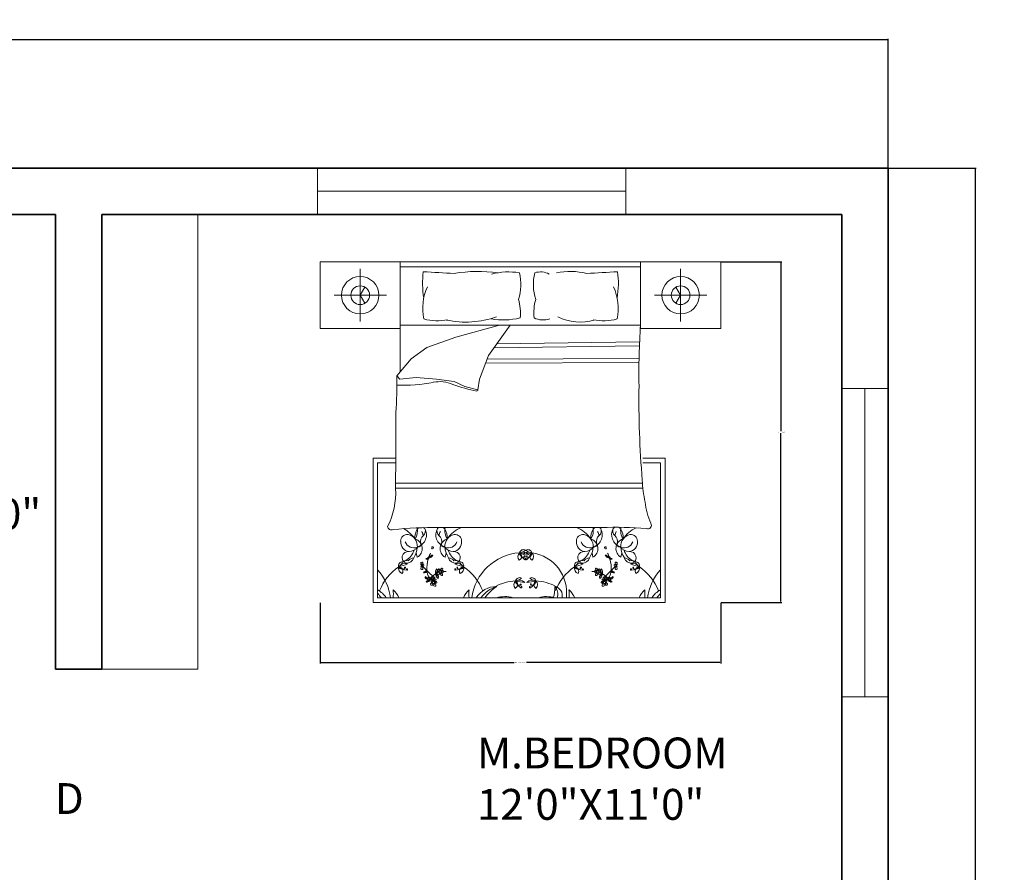
# Model space of a CAD drawing. Units: inches. Extents: x -43 to 1296, y -568 to 542.
# Tile 4 of 14: x 220 to 411, y -130 to 36. Entities that reach past the tile are written whole.
import ezdxf

# ---------------------------------------------------------------- set-up
doc = ezdxf.new("R2010")
doc.units = ezdxf.units.IN
doc.header["$MEASUREMENT"] = 0
for name, color, linetype, lineweight in [('A-ANNO-DIMS', 2, 'Continuous', 18), ('A-ANNO-TEXT', 7, 'Continuous', 18), ('A-AREA-IDEN', 7, 'Continuous', 18), ('A-FLOR-CASE', 9, 'Continuous', 18), ('A-FURN', 8, 'Continuous', 13), ('A-GLAZ', 6, 'Continuous', 18), ('A-WALL', 7, 'Continuous', 35)]:
    doc.layers.add(name, color=color, linetype=linetype, lineweight=lineweight)
doc.styles.get("Standard").update_dxf_attribs({"font": 'arial.ttf'})
doc.dimstyles.get("Standard").update_dxf_attribs({"dimtxt": 0.18, "dimasz": 0.18, "dimexe": 0.18, "dimexo": 0.0625, "dimgap": 0.09, "dimtad": 0, "dimtih": 1, "dimtoh": 1, "dimdec": 0, "dimzin": 0, "dimdsep": 46, "dimlunit": 3, "dimtxsty": 'Standard', "dimcen": 0.09, "dimadec": 0, "dimazin": 0, "dimtfac": 1, "dimtdec": 0, "dimtofl": 0, "dimtmove": 0, "dimatfit": 3, "dimfxl": 1, "dimtolj": 1, "dimtzin": 0, "dimarcsym": 0})

# ---------------------------------------------------------------- blocks, each defined once
blk = doc.blocks.new('*D1')
at = {"layer": 'A-ANNO-DIMS', "color": 0, "lineweight": -2, "transparency": 16777216}
for p, q in [((28.84, 6.72), (28.84, 31.8)), ((29.02, 31.62), (203.66, 31.62)), ((388.66, 31.62), (214.02, 31.62)), ((388.84, 6.72), (388.84, 31.8))]:
    blk.add_line(p, q, dxfattribs=at)
at = {"layer": 'A-ANNO-DIMS', "color": 0, "transparency": 16777216}
for points in [[(29.02, 31.65), (29.02, 31.59), (28.84, 31.62)], [(388.66, 31.65), (388.66, 31.59), (388.84, 31.62)]]:
    blk.add_solid(points, dxfattribs=at)
at = {"layer": 'Defpoints', "color": 0, "transparency": 16777216}
for p in [(388.84, 31.62), (28.84, 6.66), (388.84, 6.66)]:
    blk.add_point(p, dxfattribs=at)
at = {"layer": 'A-ANNO-DIMS', "color": 0, "transparency": 16777216, "insert": (208.84, 31.62), "char_height": 6, "attachment_point": 5}
blk.add_mtext("\\A1;30'", dxfattribs=at)
blk = doc.blocks.new('*D2')
at = {"layer": 'A-ANNO-DIMS', "color": 0, "lineweight": -2, "transparency": 16777216}
for p, q in [((388.91, 6.66), (405.97, 6.66)), ((405.79, 6.48), (405.79, -230.19)), ((405.79, -473.16), (405.79, -236.49)), ((388.91, -473.34), (405.97, -473.34))]:
    blk.add_line(p, q, dxfattribs=at)
at = {"layer": 'A-ANNO-DIMS', "color": 0, "transparency": 16777216}
for points in [[(405.76, 6.48), (405.82, 6.48), (405.79, 6.66)], [(405.76, -473.16), (405.82, -473.16), (405.79, -473.34)]]:
    blk.add_solid(points, dxfattribs=at)
at = {"layer": 'Defpoints', "color": 0, "transparency": 16777216}
for p in [(388.84, 6.66), (388.84, -473.34), (405.79, -473.34)]:
    blk.add_point(p, dxfattribs=at)
at = {"layer": 'A-ANNO-DIMS', "color": 0, "transparency": 16777216, "insert": (405.79, -233.34), "char_height": 6, "attachment_point": 5}
blk.add_mtext("\\A1;40'", dxfattribs=at)
blk = doc.blocks.new('BED-SUITE-78')
for p, q in [((0, 66.29), (77.95, 66.29)), ((15.59, 66.29), (15.59, 44.89)), ((62.36, 65.29), (15.59, 65.29)), ((7.79, 54.7), (7.79, 64.89)), ((70.15, 54.7), (70.15, 64.89)), ((12.89, 59.79), (2.7, 59.79)), ((65.06, 59.79), (75.25, 59.79)), ((15.59, 53.97), (62.36, 53.97)), ((26.42, 51.65), (34.92, 53.97)), ((37, 53.97), (32.73, 48.03)), ((20.73, 49.6), (26.42, 51.65)), ((62.12, 49.93), (33.82, 49.53)), ((62.15, 50.73), (34.4, 50.34)), ((17.73, 47.39), (20.73, 49.6)), ((32.73, 48.03), (31, 43.45)), ((14.89, 44.08), (17.73, 47.39)), ((62.08, 46.68), (32.17, 46.56)), ((62.08, 47.48), (32.48, 47.36)), ((15.52, 43.45), (14.89, 44.08)), ((18.68, 43.77), (15.52, 43.45)), ((22.63, 43.45), (18.68, 43.77)), ((26.1, 42.98), (22.63, 43.45)), ((28.15, 42.03), (26.1, 42.98)), ((31, 43.45), (30.68, 41.4)), ((30.68, 41.4), (28.15, 42.03)), ((10.29, 28.08), (14.7, 28.08)), ((10.29, 0), (10.29, 28.08)), ((14.7, 27.18), (11.19, 27.18)), ((11.19, 27.18), (11.19, 0.9)), ((66.21, 27.18), (62.78, 27.18)), ((62.79, 28.08), (67.12, 28.08)), ((66.21, 0.9), (66.21, 27.18)), ((67.12, 28.08), (67.12, 0)), ((62.71, 23.22), (14.69, 23.22)), ((62.79, 22.25), (14.69, 22.25)), ((54.8, 14.59), (23.15, 14.59)), ((18.87, 8.81), (18.7, 9.69)), ((24.32, 8.81), (24.49, 9.69)), ((53.08, 8.81), (52.91, 9.69)), ((58.53, 8.81), (58.7, 9.69)), ((67.12, 0), (10.29, 0)), ((11.19, 0.9), (66.21, 0.9))]:
    blk.add_line(p, q)
for points in [[(15.59, 53.3), (0, 53.3), (0, 66.29)], [(62.36, 66.29), (62.36, 53.3), (77.95, 53.3), (77.95, 66.29)], [(7.79, 59.79), (8.7, 61.37)], [(70.15, 59.79), (69.24, 61.37)], [(7.79, 59.79), (8.7, 58.22)], [(70.15, 59.79), (69.24, 58.22)]]:
    blk.add_lwpolyline(points)
for points in [[(20.07, 64.35, 0.074897), (20.16, 59.26, -0.472817)], [(38.61, 58.97, 0.14099), (38.76, 64.16, 0.235245)], [(41.94, 58.97, -0.14099), (41.78, 64.16, -0.235245)], [(57.88, 64.35, -0.074897), (57.79, 59.26, 0.472817)], [(14.73, 36.94, 0.001242), (14.69, 22.15, -0.127202), (13.13, 14.78)], [(62.69, 23.83, 0.056112), (63.26, 19.54, 0.095341), (64.35, 15.41)]]:
    blk.add_lwpolyline(points, format="xyb")
for centre, radius in [((7.79, 59.79), 3.64), ((70.15, 59.79), 3.64), ((7.79, 59.79), 1.82), ((70.15, 59.79), 1.82), ((23.38, 5.98), 0.199), ((54.03, 5.98), 0.199), ((22.08, 3.89), 0.199), ((55.33, 3.89), 0.199)]:
    blk.add_circle(centre, radius)
for centre, radius, start, end in [((63.03, 806.15), 743.04, 266.68521, 267.14978), ((30.75, 36.14), 28.27, 82.2196, 99.497), ((36.72, 50.43), 13.89, 81.5249, 103.96), ((42.85, 60.46), 3.86, 63.3437, 106.1026), ((48.63, 50.71), 13.7, 76.3427, 101.1841), ((14.92, 806.15), 743.04, 272.85022, 273.31479), ((30, 57.21), 10.05, 155.1316, 191.7583), ((47.95, 57.21), 10.05, 348.2417, 24.8684), ((29.42, 56.37), 9.55, 354.0129, 15.8293), ((51.13, 56.37), 9.55, 164.1707, 185.9871), ((28.35, 72.68), 18.12, 258.0397, 289.2615), ((50.59, 64.49), 9.92, 243.8761, 286.1746), ((22.85, 65.26), 10.45, 255.1039, 281.0369), ((35.68, 68.73), 13.75, 259.8617, 283.6238), ((43.37, 59.11), 4.13, 245.0183, 288.5407), ((55.1, 65.26), 10.45, 258.9631, 284.8961), ((202.09, 44.45), 140.06, 176.1, 180.9282), ((-56.58, 42.14), 71.5, 355.8294, 1.553), ((16.23, 71.68), 29.42, 267.4519, 281.3392), ((23.26, 36.62), 6.35, 66.2616, 101.3392), ((36.09, 70.85), 30.23, 250.1194, 259.3383), ((244.73, 39.35), 182.7, 179.1145, 184.8735), ((30.5, 41.34), 0.188, 268.8623, 19.7536), ((63.76, 15.02), 0.71, 246.5219, 33.8264), ((13.85, 14.83), 0.719, 183.98, 297.3412), ((22.22, -66.55), 81.14, 89.3433, 95.6887), ((13.54, 9.1), 5.9, 33.6671, 63.2997), ((21.45, 12.61), 3.01, 145.785, 184.7304), ((15.71, 14.01), 3.23, 328.8218, 9.1554), ((19.71, 13.73), 0.939, 120.0293, 142.325), ((18.21, 13.17), 2.48, 289.2822, 29.1751), ((17.83, 12.72), 2.24, 7.436, 29.9149), ((19.31, 13.91), 1.17, 311.5653, 23.8354), ((19.71, 13.73), 0.939, 44.4517, 63.558), ((24.99, 13.17), 2.48, 150.8249, 250.7178), ((23.88, 13.91), 1.17, 156.1646, 228.4347), ((23.49, 13.73), 0.939, 113.229, 135.5483), ((25.36, 12.72), 2.24, 150.0851, 172.564), ((23.49, 13.73), 0.939, 37.675, 66.7144), ((21.74, 12.61), 3.01, 355.2696, 34.215), ((27.49, 14.01), 3.23, 169.7133, 211.1782), ((29.65, 9.1), 5.9, 111.4941, 146.3329), ((47.75, 9.1), 5.9, 33.6671, 68.5059), ((55.66, 12.61), 3.01, 145.785, 184.7304), ((49.92, 14.01), 3.23, 328.8218, 10.2867), ((53.92, 13.73), 0.939, 113.2856, 142.325), ((52.42, 13.17), 2.48, 289.2822, 29.1751), ((52.04, 12.72), 2.24, 7.436, 29.9149), ((53.92, 13.73), 0.939, 44.4517, 66.7144), ((53.52, 13.91), 1.17, 311.5653, 23.8354), ((57.18, -61.22), 75.85, 85.2402, 91.8035), ((59.2, 13.17), 2.48, 150.8249, 250.7178), ((58.09, 13.91), 1.17, 156.1646, 228.4347), ((57.7, 13.73), 0.939, 106.6343, 135.5483), ((59.57, 12.72), 2.24, 150.0851, 172.564), ((57.7, 13.73), 0.939, 37.675, 72.5814), ((55.96, 12.61), 3.01, 355.2696, 34.215), ((61.7, 14.01), 3.23, 169.249, 211.1782), ((63.86, 9.1), 5.9, 113.6453, 146.3329), ((16.98, 11.93), 1.32, 84.4856, 181.0538), ((17.52, 11.74), 1.86, 174.9449, 262.8857), ((18.25, 12.45), 1.81, 201.5819, 291.4221), ((16.58, 10.96), 2.34, 355.2933, 76.921), ((17.91, 10.49), 1.94, 299.9085, 73.1337), ((21.14, 11.84), 1.6, 131.5653, 195.1471), ((22.05, 11.84), 1.6, 344.8529, 48.4347), ((25.29, 10.49), 1.94, 106.8663, 240.0915), ((26.62, 10.96), 2.34, 103.079, 184.7067), ((24.94, 12.45), 1.81, 248.5779, 338.4181), ((25.68, 11.74), 1.86, 277.1143, 5.0551), ((26.21, 11.93), 1.32, 358.9462, 95.5144), ((51.19, 11.93), 1.32, 84.4856, 181.0538), ((51.73, 11.74), 1.86, 174.9449, 262.8857), ((52.46, 12.45), 1.81, 201.5819, 291.4221), ((50.79, 10.96), 2.34, 355.2933, 76.921), ((52.12, 10.49), 1.94, 299.9085, 73.1337), ((55.35, 11.84), 1.6, 131.5653, 195.1471), ((56.26, 11.84), 1.6, 344.8529, 48.4347), ((59.5, 10.49), 1.94, 106.8663, 240.0915), ((60.83, 10.96), 2.34, 103.079, 184.7067), ((59.15, 12.45), 1.81, 248.5779, 338.4181), ((59.89, 11.74), 1.86, 277.1143, 5.0551), ((60.42, 11.93), 1.32, 358.9462, 95.5144), ((17.09, 8.74), 1.17, 80.264, 250.8688), ((14.77, 11.32), 3.68, 301.2614, 341.7045), ((17.19, 12.16), 2.26, 272.3591, 324.0401), ((14.74, 11.02), 4.18, 326.2883, 356.5076), ((21.45, 12.61), 3.01, 212.7011, 216.3445), ((19.13, 11.3), 0.484, 257.3041, 15.1471), ((21.82, 10.57), 0.15, 102.7051, 280.4384), ((21.8, 10.66), 0.244, 280.4384, 100.4136), ((24.06, 11.3), 0.484, 164.8529, 282.6959), ((21.74, 12.61), 3.01, 323.6555, 327.2989), ((26, 12.16), 2.26, 215.9599, 267.6409), ((28.46, 11.02), 4.18, 183.4924, 213.7117), ((28.42, 11.32), 3.68, 198.2955, 238.7386), ((26.1, 8.74), 1.17, 289.1312, 99.736), ((39.58, -0.47), 10.18, 94.4623, 172.255), ((39.62, 8.92), 1.13, 137.7873, 219.1145), ((38.34, 8.96), 0.85, 298.5391, 58.3627), ((39.6, 9.44), 0.844, 63.0274, 163.8037), ((38.74, 11.42), 1.74, 271.4585, 315.3727), ((39.45, 8.21), 1.61, 45.5411, 114.3101), ((40.92, 16.47), 7.12, 252.593, 267.2582), ((39.62, 9.65), 0.833, 177.7585, 283.852), ((41.22, 10.51), 2.57, 198.9159, 238.011), ((40.55, 8.21), 1.61, 65.6899, 134.4589), ((39.08, 16.47), 7.12, 272.7418, 287.407), ((40.4, 9.44), 0.844, 16.1963, 116.9726), ((41.26, 11.42), 1.74, 224.6273, 268.5415), ((38.78, 10.51), 2.57, 301.989, 341.0841), ((40.38, 9.65), 0.833, 256.148, 2.2415), ((41.66, 8.96), 0.85, 121.6373, 241.4609), ((40.38, 8.92), 1.13, 320.8855, 42.2127), ((40.09, 1.88), 7.88, 352.8636, 81.8197), ((51.3, 8.74), 1.17, 80.264, 250.8688), ((48.98, 11.32), 3.68, 301.2614, 341.7045), ((51.4, 12.16), 2.26, 272.3591, 324.0401), ((48.95, 11.02), 4.18, 326.2883, 356.5076), ((55.66, 12.61), 3.01, 212.7011, 216.3445), ((53.34, 11.3), 0.484, 257.3041, 15.1471), ((55.6, 10.66), 0.244, 79.5864, 259.5616), ((55.58, 10.57), 0.15, 259.5616, 77.2949), ((58.27, 11.3), 0.484, 164.8529, 282.6959), ((55.96, 12.61), 3.01, 323.6555, 327.2989), ((60.21, 12.16), 2.26, 215.9599, 267.6409), ((62.67, 11.02), 4.18, 183.4924, 213.7117), ((62.63, 11.32), 3.68, 198.2955, 238.7386), ((60.31, 8.74), 1.17, 289.1312, 99.736), ((16.1, 7.13), 0.844, 92.9516, 193.728), ((14.37, 8.41), 1.74, 301.3827, 345.2969), ((16.85, 7.48), 0.717, 63.9755, 143.2681), ((16.81, 9.09), 1.46, 265.969, 344.3045), ((18.38, 7.15), 1.56, 96.1662, 141.5825), ((19.8, 7.47), 0.331, 101.5637, 142.6358), ((19.54, 7.73), 0.477, 288.7263, 352.5032), ((19.86, 7.7), 0.153, 345.2356, 144.9248), ((20.96, 8.24), 0.409, 101.3256, 154.4621), ((20.37, 9.63), 1.23, 280.2588, 300.656), ((20.65, 10.62), 2.2, 268.3264, 277.1302), ((27.22, 6.64), 6.46, 163.5842, 183.8277), ((20.1, 9.63), 1.25, 308.2101, 316.3071), ((20.87, 8.81), 0.374, 278.3432, 4.2869), ((20.67, 9.14), 0.653, 300.656, 332.6341), ((21.16, 8.7), 0.159, 55.7657, 157.4417), ((27.22, 6.64), 6.46, 153.0032, 159.8941), ((21.4, 8.85), 0.159, 84.3784, 186.0543), ((21.26, 9.49), 0.653, 269.1859, 301.164), ((21.45, 9.15), 0.374, 237.5332, 323.4768), ((21.08, 10.22), 1.25, 285.5129, 293.6099), ((20.96, 9.98), 1.23, 301.164, 321.5612), ((21.9, 8.81), 0.409, 87.3579, 140.4944), ((19.95, 10.2), 2.2, 324.6898, 333.4936), ((24.81, 7.15), 1.56, 38.4175, 83.8338), ((26.38, 9.09), 1.46, 195.6955, 274.031), ((26.34, 7.48), 0.717, 36.7319, 116.0245), ((27.09, 7.13), 0.844, 346.272, 87.0484), ((28.82, 8.41), 1.74, 194.7031, 238.6173), ((39.79, 8.95), 0.11, 283.852, 219.9245), ((39.93, 8.44), 0.126, 238.011, 71.5592), ((39.95, 8.5), 0.0614, 71.5592, 188.0167), ((40.08, 8.44), 0.126, 108.4408, 301.989), ((40.06, 8.5), 0.0614, 351.9833, 108.4408), ((40.2, 8.99), 0.0664, 320.1909, 256.0209), ((50.31, 7.13), 0.844, 92.9516, 193.728), ((48.58, 8.41), 1.74, 301.3827, 345.2969), ((51.06, 7.48), 0.717, 63.9755, 143.2681), ((51.02, 9.09), 1.46, 265.969, 344.3045), ((52.59, 7.15), 1.56, 96.1662, 141.5825), ((56.45, 9.98), 1.23, 218.4388, 238.836), ((55.5, 8.81), 0.409, 39.5056, 92.6421), ((57.45, 10.2), 2.2, 206.5064, 215.3102), ((55.96, 9.15), 0.374, 216.5232, 302.4668), ((56.15, 9.49), 0.653, 238.836, 270.8141), ((56.32, 10.22), 1.25, 246.3901, 254.4871), ((50.18, 6.64), 6.46, 20.1059, 26.9968), ((56, 8.85), 0.159, 353.9457, 95.6216), ((56.25, 8.7), 0.159, 22.5583, 124.2343), ((56.53, 8.81), 0.374, 175.7131, 261.6568), ((56.74, 9.14), 0.653, 207.3659, 239.344), ((50.18, 6.64), 6.46, 356.1723, 16.4158), ((57.3, 9.63), 1.25, 223.6929, 231.7899), ((57.03, 9.63), 1.23, 239.344, 259.7412), ((56.75, 10.62), 2.2, 262.8698, 271.6736), ((56.44, 8.24), 0.409, 25.5379, 78.6744), ((57.54, 7.7), 0.153, 35.0752, 194.7644), ((57.87, 7.73), 0.477, 187.4968, 251.2737), ((57.6, 7.47), 0.331, 37.3642, 78.4363), ((60.59, 9.09), 1.46, 195.6955, 274.031), ((59.02, 7.15), 1.56, 38.4175, 83.8338), ((60.55, 7.48), 0.717, 36.7319, 116.0245), ((63.03, 8.41), 1.74, 194.7031, 238.6173), ((61.3, 7.13), 0.844, 346.272, 87.0484), ((3.61, -0.47), 10.18, 7.745, 41.8856), ((21.03, -1.47), 10.18, 124.3865, 158.5908), ((16.38, 6.69), 1.13, 167.7115, 249.0387), ((16.59, 5.98), 1.61, 75.4653, 144.2343), ((13.74, 13.88), 7.12, 282.5173, 297.1824), ((15.25, 6.08), 0.85, 328.4633, 88.2869), ((16.97, 8.86), 2.57, 228.8402, 267.9352), ((16.02, 7.31), 0.833, 207.6827, 313.7762), ((16.52, 6.79), 0.11, 313.7762, 249.7183), ((16.87, 6.48), 0.0614, 101.4834, 217.9409), ((16.89, 6.42), 0.126, 267.9352, 101.4834), ((19.53, 7.16), 0.199, 273.2768, 86.7232), ((19.8, 6.79), 0.328, 217.7621, 259.0403), ((19.76, 7.35), 0.19, 91.1081, 181.8675), ((20.15, 7.23), 0.603, 203.4276, 227.6104), ((19.96, 6.97), 0.41, 80.3487, 133.6538), ((19.89, 7.31), 0.325, 229.7889, 317.6792), ((19.52, 6.62), 0.461, 355.053, 68.3618), ((19.88, 6.54), 0.65, 83.0852, 105.7171), ((19.83, 6.59), 0.152, 232.4737, 355.053), ((15.38, 1.15), 7.4, 43.1541, 52.0459), ((20, 7.2), 0.171, 317.6792, 80.3487), ((20.5, 5.62), 0.409, 101.3256, 154.4621), ((19.91, 7.01), 1.23, 280.2588, 300.656), ((20.19, 8), 2.2, 268.3264, 277.1302), ((19.64, 7.01), 1.25, 308.2101, 316.3071), ((20.41, 6.18), 0.374, 278.3432, 4.2869), ((20.2, 6.51), 0.653, 300.656, 332.6341), ((20.69, 6.08), 0.159, 55.7657, 157.4417), ((24.01, 6.48), 3.24, 184.756, 209.2041), ((28.67, 13.37), 10.65, 222.2412, 232.1744), ((21.86, 6.28), 0.905, 304.5369, 16.3699), ((22.34, 6.07), 0.55, 272.8499, 356.1226), ((21.95, 5.86), 0.533, 321.7607, 7.9252), ((23.11, 6.02), 0.64, 127.3105, 187.9252), ((22.23, 6.09), 0.657, 355.0106, 41.658), ((24.34, 2.18), 3.88, 113.0501, 113.8477), ((23.32, 5.38), 0.626, 104.7558, 148.0499), ((22.97, 5.83), 0.392, 247.4086, 351.4386), ((23.16, 6.26), 0.271, 126.1046, 271.4281), ((23.13, 6.33), 0.194, 353.7526, 131.7054), ((23.08, 5.81), 0.131, 262.906, 7.132), ((22.94, 6.1), 0.273, 0.0645, 61.1507), ((23.01, 6.33), 0.312, 311.8413, 355.7877), ((23.65, 6.29), 0.331, 101.5637, 176.365), ((23.65, 5.61), 0.328, 151.2196, 259.0403), ((23.61, 6.17), 0.19, 91.1081, 181.8675), ((24, 6.05), 0.603, 203.4276, 227.6104), ((23.81, 5.79), 0.41, 80.3487, 133.6538), ((23.74, 6.13), 0.325, 229.7889, 317.6792), ((23.38, 6.55), 0.477, 288.7263, 352.5032), ((23.37, 5.44), 0.461, 355.053, 68.3618), ((23.73, 5.36), 0.65, 83.0852, 105.7171), ((23.71, 6.53), 0.153, 345.2356, 144.9248), ((23.85, 6.02), 0.171, 317.6792, 80.3487), ((24.34, 2.18), 3.88, 87.1071, 94.7585), ((26.31, 6.42), 0.126, 78.5166, 272.0648), ((26.61, 5.98), 1.61, 35.7657, 104.5347), ((29.46, 13.88), 7.12, 242.8176, 257.4827), ((26.22, 8.86), 2.57, 272.0648, 311.1598), ((26.32, 6.48), 0.0614, 322.0591, 78.5166), ((27.18, 7.31), 0.833, 226.2238, 332.3173), ((26.69, 6.83), 0.0664, 290.2667, 226.2271), ((27.94, 6.08), 0.85, 91.7131, 211.5367), ((26.81, 6.69), 1.13, 290.9613, 12.2885), ((22.17, -1.47), 10.18, 21.4092, 55.6135), ((55.24, -1.47), 10.18, 124.3865, 158.5908), ((50.59, 6.69), 1.13, 167.7115, 249.0387), ((50.8, 5.98), 1.61, 75.4653, 144.2343), ((47.95, 13.88), 7.12, 282.5173, 297.1824), ((50.23, 7.31), 0.833, 207.6827, 313.7762), ((51.18, 8.86), 2.57, 228.8402, 267.9352), ((49.46, 6.08), 0.85, 328.4633, 88.2869), ((50.73, 6.79), 0.11, 313.7762, 249.7183), ((51.08, 6.48), 0.0614, 101.4834, 217.9409), ((51.1, 6.42), 0.126, 267.9352, 101.4834), ((53.06, 2.18), 3.88, 85.2415, 92.8929), ((53.55, 6.02), 0.171, 99.6513, 222.3208), ((53.67, 6.13), 0.325, 222.3208, 310.2111), ((53.59, 5.79), 0.41, 46.3462, 99.6513), ((53.69, 6.53), 0.153, 35.0752, 194.7644), ((54.02, 6.55), 0.477, 187.4968, 251.2737), ((54.03, 5.44), 0.461, 111.6382, 184.947), ((53.67, 5.36), 0.65, 74.2829, 96.9148), ((53.8, 6.17), 0.19, 358.1325, 88.8919), ((53.4, 6.05), 0.603, 312.3896, 336.5724), ((53.75, 6.29), 0.331, 3.635, 78.4363), ((53.76, 5.61), 0.328, 280.9597, 28.7804), ((54.43, 5.83), 0.392, 188.5614, 292.5914), ((54.28, 6.33), 0.194, 48.2946, 186.2474), ((54.39, 6.33), 0.312, 184.2123, 228.1587), ((54.46, 6.1), 0.273, 118.8493, 179.9355), ((54.32, 5.81), 0.131, 172.868, 277.094), ((54.25, 6.26), 0.271, 268.5719, 53.8954), ((54.08, 5.38), 0.626, 31.9501, 75.2442), ((55.17, 6.09), 0.657, 138.342, 184.9894), ((55.06, 6.07), 0.55, 183.8774, 267.1501), ((53.06, 2.18), 3.88, 66.1523, 66.9499), ((55.55, 6.28), 0.905, 163.6301, 235.4631), ((54.29, 6.02), 0.64, 352.0748, 52.6895), ((55.45, 5.86), 0.533, 172.0748, 218.2393), ((48.74, 13.37), 10.65, 307.8256, 317.7588), ((53.4, 6.48), 3.24, 330.7959, 355.244), ((62.02, 1.15), 7.4, 127.9541, 136.8459), ((56.71, 6.08), 0.159, 22.5583, 124.2343), ((57, 6.18), 0.374, 175.7131, 261.6568), ((57.2, 6.51), 0.653, 207.3659, 239.344), ((57.76, 7.01), 1.25, 223.6929, 231.7899), ((57.5, 7.01), 1.23, 239.344, 259.7412), ((57.21, 8), 2.2, 262.8698, 271.6736), ((56.91, 5.62), 0.409, 25.5379, 78.6744), ((57.4, 7.2), 0.171, 99.6513, 222.3208), ((57.52, 7.31), 0.325, 222.3208, 310.2111), ((57.44, 6.97), 0.41, 46.3462, 99.6513), ((57.88, 6.62), 0.461, 111.6382, 184.947), ((57.57, 6.59), 0.152, 184.947, 307.5263), ((57.52, 6.54), 0.65, 74.2829, 96.9148), ((57.64, 7.35), 0.19, 358.1325, 88.8919), ((57.25, 7.23), 0.603, 312.3896, 336.5724), ((57.61, 6.79), 0.328, 280.9597, 322.2379), ((57.88, 7.16), 0.199, 93.2768, 266.7232), ((60.52, 6.42), 0.126, 78.5166, 272.0648), ((60.82, 5.98), 1.61, 35.7657, 104.5347), ((63.67, 13.88), 7.12, 242.8176, 257.4827), ((60.43, 8.86), 2.57, 272.0648, 311.1598), ((60.53, 6.48), 0.0614, 322.0591, 78.5166), ((61.39, 7.31), 0.833, 226.2238, 332.3173), ((60.9, 6.83), 0.0664, 290.2667, 226.2271), ((62.15, 6.08), 0.85, 91.7131, 211.5367), ((61.02, 6.69), 1.13, 290.9613, 12.2885), ((56.38, -1.47), 10.18, 21.4092, 55.6135), ((73.79, -0.47), 10.18, 138.1144, 172.255), ((20.63, 4.9), 0.222, 146.8636, 236.9021), ((23.76, 9.79), 5.8, 235.1882, 238.8844), ((21.01, 5.22), 0.6, 199.4799, 267.6828), ((20.95, 5), 0.517, 212.8155, 277.3992), ((20.65, 4.65), 0.6, 266.9701, 338.2913), ((17.48, 8.93), 5.8, 302.6784, 306.3746), ((20.8, 4.18), 0.222, 214.3538, 304.3923), ((20.88, 5.02), 0.229, 238.8844, 314.2646), ((20.83, 4.5), 0.517, 280.3057, 17.1958), ((20.79, 4.45), 0.229, 306.3746, 21.7548), ((21.16, 4.6), 0.173, 19.3605, 201.7548), ((21.16, 4.73), 0.173, 311.8703, 134.2646), ((24.42, 3.15), 3.46, 153.7819, 158.2913), ((21.66, 5.51), 0.905, 247.2305, 319.0635), ((21.37, 5.21), 0.533, 264.4544, 310.6188), ((24.01, 6.48), 3.24, 214.0033, 222.4917), ((21.76, 5), 0.55, 218.3208, 298.8162), ((24.34, 2.18), 3.88, 120.544, 139.818), ((22.02, 3.29), 0.626, 104.7558, 148.0499), ((21.86, 4.17), 0.271, 126.1046, 271.4281), ((21.83, 4.24), 0.194, 353.7526, 131.7054), ((22.13, 4.32), 0.64, 70.0041, 130.6188), ((21.65, 4.01), 0.273, 0.0645, 61.1507), ((21.71, 4.24), 0.312, 311.8413, 355.7877), ((21.71, 5.1), 0.657, 297.7043, 344.3516), ((22.35, 4.2), 0.331, 101.5637, 176.365), ((22.31, 4.08), 0.19, 91.1081, 181.8675), ((22.51, 3.7), 0.41, 80.3487, 133.6538), ((22.09, 4.46), 0.477, 288.7263, 352.5032), ((22.43, 3.27), 0.65, 83.0852, 105.7171), ((22.41, 4.43), 0.153, 345.2356, 144.9248), ((22.06, 5.1), 0.533, 8.7227, 54.8872), ((22.09, 4.67), 0.905, 0.278, 72.111), ((22.5, 5), 0.55, 20.5253, 88.5375), ((22.55, 3.93), 0.171, 317.6792, 80.3487), ((23.22, 5.27), 0.64, 188.7227, 249.3375), ((22.96, 5.61), 0.197, 148.0499, 225.6268), ((22.4, 4.95), 0.657, 334.9899, 21.6373), ((23.68, 5.41), 0.152, 232.4737, 355.053), ((38.8, -5.92), 10.18, 94.4623, 117.4146), ((38.84, 3.47), 1.13, 137.7873, 219.1145), ((37.56, 3.5), 0.85, 298.5391, 58.3627), ((38.82, 3.99), 0.844, 63.0274, 163.8037), ((37.96, 5.97), 1.74, 271.4585, 315.3727), ((38.67, 2.76), 1.61, 45.5411, 114.3101), ((40.44, 5.06), 2.57, 198.9159, 238.011), ((40.14, 11.02), 7.12, 252.593, 267.2582), ((38.84, 4.2), 0.833, 177.7585, 283.852), ((41.33, 2.76), 1.61, 65.6899, 134.4589), ((39.86, 11.02), 7.12, 272.7418, 287.407), ((41.18, 3.99), 0.844, 16.1963, 116.9726), ((42.04, 5.97), 1.74, 224.6273, 268.5415), ((39.56, 5.06), 2.57, 301.989, 341.0841), ((41.16, 4.2), 0.833, 256.148, 2.2415), ((42.44, 3.5), 0.85, 121.6373, 241.4609), ((41.16, 3.47), 1.13, 320.8855, 42.2127), ((41.2, -5.92), 10.18, 62.5854, 85.5377), ((53.73, 5.41), 0.152, 184.947, 307.5263), ((55, 4.95), 0.657, 158.3627, 205.0101), ((54.91, 5), 0.55, 91.4625, 159.4747), ((55.31, 4.67), 0.905, 107.889, 179.722), ((54.18, 5.27), 0.64, 290.6625, 351.2773), ((54.44, 5.61), 0.197, 314.3732, 31.9501), ((54.85, 3.93), 0.171, 99.6513, 222.3208), ((55.34, 5.1), 0.533, 125.1128, 171.2773), ((54.89, 3.7), 0.41, 46.3462, 99.6513), ((54.99, 4.43), 0.153, 35.0752, 194.7644), ((55.32, 4.46), 0.477, 187.4968, 251.2737), ((54.97, 3.27), 0.65, 74.2829, 96.9148), ((53.06, 2.18), 3.88, 40.182, 59.456), ((55.27, 4.32), 0.64, 49.3812, 109.9959), ((55.74, 5.51), 0.905, 220.9365, 292.7695), ((55.69, 5.1), 0.657, 195.6484, 242.2957), ((55.09, 4.08), 0.19, 358.1325, 88.8919), ((55.05, 4.2), 0.331, 3.635, 78.4363), ((55.65, 5), 0.55, 241.1838, 321.6792), ((55.58, 4.24), 0.194, 48.2946, 186.2474), ((55.69, 4.24), 0.312, 184.2123, 228.1587), ((55.76, 4.01), 0.273, 118.8493, 179.9355), ((55.55, 4.17), 0.271, 268.5719, 53.8954), ((55.38, 3.29), 0.626, 31.9501, 75.2442), ((56.04, 5.21), 0.533, 229.3812, 275.5456), ((53.4, 6.48), 3.24, 317.5083, 325.9967), ((56.57, 4.5), 0.517, 162.8042, 259.6943), ((56.24, 4.73), 0.173, 45.7354, 228.1297), ((56.24, 4.6), 0.173, 338.2452, 160.6395), ((52.99, 3.15), 3.46, 21.7087, 26.2181), ((56.76, 4.65), 0.6, 201.7087, 273.0299), ((56.52, 5.02), 0.229, 225.7354, 301.1156), ((56.46, 5), 0.517, 262.6008, 327.1845), ((56.62, 4.45), 0.229, 158.2452, 233.6254), ((56.39, 5.22), 0.6, 272.3172, 340.5201), ((59.92, 8.93), 5.8, 233.6254, 237.3216), ((56.61, 4.18), 0.222, 235.6077, 325.6462), ((53.65, 9.79), 5.8, 301.1156, 304.8118), ((56.77, 4.9), 0.222, 303.0979, 33.1364), ((8.72, -1.83), 4.96, 33.4617, 60.1116), ((11.5, -0.68), 4.14, 22.5547, 48.9546), ((0.16, 1.54), 14.08, 357.4081, 3.6519), ((21.66, 3.52), 0.197, 148.0499, 225.6268), ((21.67, 3.74), 0.392, 247.4086, 351.4386), ((21.78, 3.72), 0.131, 262.906, 7.132), ((22.35, 3.52), 0.328, 151.2196, 259.0403), ((22.7, 3.96), 0.603, 203.4276, 227.6104), ((22.44, 4.04), 0.325, 229.7889, 317.6792), ((22.07, 3.35), 0.461, 355.053, 68.3618), ((22.38, 3.32), 0.152, 232.4737, 355.053), ((31.7, -0.68), 4.14, 131.0454, 157.4453), ((43.03, 1.54), 14.08, 176.3481, 182.5919), ((34.47, -1.83), 4.96, 91.272, 146.5383), ((36.26, -2.76), 6.18, 107.8504, 143.6964), ((39.51, -4.49), 9.19, 124.0123, 144.053), ((39.01, 3.49), 0.11, 283.852, 219.9245), ((39.15, 2.99), 0.126, 238.011, 71.5592), ((39.17, 3.05), 0.0614, 71.5592, 188.0167), ((40.86, 2.99), 0.126, 108.4408, 301.989), ((40.83, 3.05), 0.0614, 351.9833, 108.4408), ((40.98, 3.54), 0.0664, 320.1909, 256.0209), ((41.11, 2.6), 4.56, 338.117, 6.6195), ((45.29, 1.33), 1.83, 346.3898, 79.0739), ((43.92, 1.58), 2.31, 342.8609, 41.9049), ((34.37, 1.54), 14.08, 357.4081, 3.6519), ((45.71, -0.68), 4.14, 22.5547, 48.9546), ((54.97, 4.04), 0.325, 222.3208, 310.2111), ((55.33, 3.35), 0.461, 111.6382, 184.947), ((55.03, 3.32), 0.152, 184.947, 307.5263), ((54.7, 3.96), 0.603, 312.3896, 336.5724), ((55.06, 3.52), 0.328, 280.9597, 28.7804), ((55.73, 3.74), 0.392, 188.5614, 292.5914), ((55.62, 3.72), 0.131, 172.868, 277.094), ((55.74, 3.52), 0.197, 314.3732, 31.9501), ((65.91, -0.68), 4.14, 131.0454, 157.4453), ((77.24, 1.54), 14.08, 176.3481, 182.5919), ((68.68, -1.83), 4.96, 119.8884, 146.5383), ((6.94, -2.76), 6.18, 36.3036, 46.4814), ((35.95, -4.45), 5.6, 73.5431, 107.0202), ((38.17, -7.33), 8.28, 94.3787, 95.6357), ((42.53, -13), 14.79, 109.7217, 109.9028), ((44.05, -4.45), 5.6, 72.9798, 106.4569), ((41.83, -7.33), 8.28, 84.3643, 85.6213), ((37.47, -13), 14.79, 70.0972, 70.2783), ((70.47, -2.76), 6.18, 133.5186, 143.6964)]:
    blk.add_arc(centre, radius, start, end)
blk = doc.blocks.new('WIN-60x9')
for p, q in [((0, 60), (0, 0)), ((9, 60), (0, 60)), ((4.5, 60), (4.5, 0)), ((9, 0), (9, 60)), ((0, 0), (9, 0))]:
    blk.add_line(p, q)
blk = doc.blocks.new('*D38')
at = {"layer": 'A-ANNO-DIMS', "color": 0, "lineweight": -2, "transparency": 16777216}
for p, q in [((278.33, -77.9), (278.33, -89.71)), ((356.28, -77.9), (356.28, -89.71)), ((278.51, -89.53), (316.1, -89.53)), ((356.1, -89.53), (318.51, -89.53))]:
    blk.add_line(p, q, dxfattribs=at)
at = {"layer": 'A-ANNO-DIMS', "color": 0, "transparency": 16777216}
for points in [[(278.51, -89.5), (278.51, -89.56), (278.33, -89.53)], [(356.1, -89.5), (356.1, -89.56), (356.28, -89.53)]]:
    blk.add_solid(points, dxfattribs=at)
at = {"layer": 'Defpoints', "color": 0, "transparency": 16777216}
for p in [(278.33, -77.84), (356.28, -77.84), (356.28, -89.53)]:
    blk.add_point(p, dxfattribs=at)
at = {"layer": 'A-ANNO-DIMS', "color": 0, "transparency": 16777216, "insert": (317.31, -89.53), "char_height": 0.18, "attachment_point": 5}
blk.add_mtext('\\A1;BED SET 6\'-6" TYP.', dxfattribs=at)
blk = doc.blocks.new('*D39')
at = {"layer": 'A-ANNO-DIMS', "color": 0, "lineweight": -2, "transparency": 16777216}
for p, q in [((356.34, -11.55), (368.15, -11.55)), ((367.97, -11.73), (367.97, -44.51)), ((367.97, -77.66), (367.97, -44.88)), ((356.34, -77.84), (368.15, -77.84))]:
    blk.add_line(p, q, dxfattribs=at)
at = {"layer": 'A-ANNO-DIMS', "color": 0, "transparency": 16777216}
for points in [[(367.94, -11.73), (368, -11.73), (367.97, -11.55)], [(367.94, -77.66), (368, -77.66), (367.97, -77.84)]]:
    blk.add_solid(points, dxfattribs=at)
at = {"layer": 'Defpoints', "color": 0, "transparency": 16777216}
for p in [(356.28, -11.55), (367.97, -11.55), (356.28, -77.84)]:
    blk.add_point(p, dxfattribs=at)
at = {"layer": 'A-ANNO-DIMS', "color": 0, "transparency": 16777216, "insert": (367.97, -44.7), "char_height": 0.18, "attachment_point": 5}
blk.add_mtext('\\A1;5\'-6 1/2" TYP.', dxfattribs=at)

msp = doc.modelspace()

# ---------------------------------------------------------------- linework, layer by layer
at = {"layer": 'A-FLOR-CASE'}
for p, q in [((254.55, -90.84), (254.55, -2.34)), ((235.84, -90.84), (254.55, -90.84))]:
    msp.add_line(p, q, dxfattribs=at)
at = {"layer": 'A-WALL'}
for p, q in [((28.84, 6.66), (388.84, 6.66)), ((388.84, 6.66), (388.84, -473.34)), ((166.84, -2.34), (226.84, -2.34)), ((226.84, -2.34), (226.84, -90.84)), ((235.84, -2.34), (235.84, -90.84)), ((235.84, -2.34), (379.84, -2.34)), ((379.84, -2.34), (379.84, -206.34)), ((226.84, -90.84), (235.84, -90.84))]:
    msp.add_line(p, q, dxfattribs=at)

# ---------------------------------------------------------------- block references
at = {"layer": 'A-FURN'}
msp.add_blockref('BED-SUITE-78', (278.33, -77.84), dxfattribs=at)
at = {"layer": 'A-GLAZ', "rotation": 270.0000000000002}
msp.add_blockref('WIN-60x9', (277.84, 6.66), dxfattribs=at)
at = {"layer": 'A-GLAZ'}
msp.add_blockref('WIN-60x9', (379.84, -96.21), dxfattribs=at)

# ---------------------------------------------------------------- texts
at = {"layer": 'A-ANNO-TEXT', "insert": (226.69, -112.99), "char_height": 6, "attachment_point": 1}
msp.add_mtext('D', dxfattribs=at)
at = {"layer": 'A-AREA-IDEN', "char_height": 6, "attachment_point": 1}
for s, insert in [('BATH\\P5\'0"X7\'0"', (188.88, -47.6)), ('M.BEDROOM\\P12\'0"X11\'0"', (308.84, -104.12))]:
    msp.add_mtext(s, dxfattribs=dict(at, insert=insert))

# ---------------------------------------------------------------- dimensions: what is measured, and where the dimension line sits
at = {"layer": 'A-ANNO-DIMS'}
dim = msp.add_linear_dim(base=(388.84, 31.62), p1=(28.84, 6.66), p2=(388.84, 6.66), dimstyle='Standard', override={"dimtxt": 6, "dimclrd": 0, "dimclre": 0, "dimclrt": 0}, dxfattribs=at)
dim.commit()
dim.dimension.update_dxf_attribs({"geometry": '*D1', "text_midpoint": (208.84, 31.62)})
dim = msp.add_linear_dim(base=(405.79, -473.34), p1=(388.84, 6.66), p2=(388.84, -473.34), angle=90, dimstyle='Standard', override={"dimtxt": 6, "dimclrd": 0, "dimclre": 0, "dimclrt": 0}, dxfattribs=at)
dim.commit()
dim.dimension.update_dxf_attribs({"geometry": '*D2', "text_midpoint": (405.79, -233.34)})
dim = msp.add_linear_dim(base=(367.97, -11.55), p1=(356.28, -77.84), p2=(356.28, -11.55), angle=90, text='<> TYP.', dimstyle='Standard', override={"dimdec": 1, "dimlfac": 1, "dimrnd": 0, "dimzin": 1, "dimdsep": 46, "dimlunit": 4, "dimfrac": 2}, dxfattribs=at)
dim.commit()
dim.dimension.update_dxf_attribs({"geometry": '*D39', "text_midpoint": (367.97, -44.7)})
dim = msp.add_linear_dim(base=(356.2806, -89.5328), p1=(278.3333, -77.8407), p2=(356.2806, -77.8407), text='BED SET <> TYP.', dimstyle='Standard', override={"dimdec": 1, "dimlfac": 1, "dimrnd": 0, "dimzin": 1, "dimdsep": 46, "dimlunit": 4, "dimfrac": 2}, dxfattribs=at)
dim.commit()
dim.dimension.update_dxf_attribs({"geometry": '*D38', "text_midpoint": (317.3069, -89.5328)})

doc.saveas('drawing.dxf')
